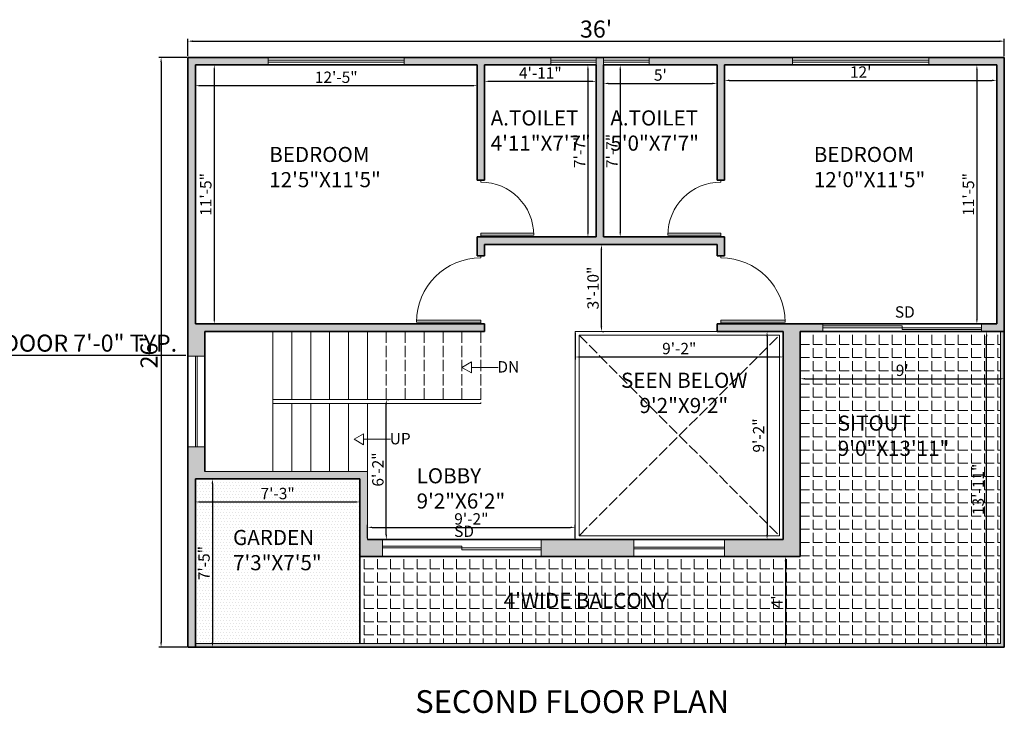
# Model space of a CAD drawing. Units: inches. Extents: x 1947 to 4744, y 610 to 1869.
# Tile 5 of 8: x 4199 to 4720, y 707 to 1074. Entities that reach past the tile are written whole.
import ezdxf

# ---------------------------------------------------------------- set-up
doc = ezdxf.new("R2010")
doc.units = ezdxf.units.IN
doc.linetypes.add('ACAD_ISO02W100', pattern=[15, 12, -3])
for name, color, linetype, lineweight in [('A-ANNO-DIMS', 2, 'Continuous', 18), ('A-ANNO-SYMB', 2, 'Continuous', 18), ('A-ANNO-TEXT', 7, 'Continuous', 18), ('A-ANNO-TITL', 7, 'Continuous', 35), ('A-AREA-IDEN', 7, 'Continuous', 18), ('A-DOOR', 3, 'Continuous', 18), ('A-FLOR-OPEN', 7, 'Continuous', 18), ('A-FLOR-OPEN-PROJ', 8, 'ACAD_ISO02W100', 13), ('A-FLOR-STRS', 7, 'Continuous', 18), ('A-FLOR-STRS-OVHD', 7, 'ACAD_ISO02W100', 13), ('A-GLAZ', 4, 'Continuous', 18), ('A-WALL', 7, 'Continuous', 35), ('A-WALL-PRHT', 7, 'Continuous', 18), ('L-PLNT-PATT', 3, 'Continuous', 13)]:
    doc.layers.add(name, color=color, linetype=linetype, lineweight=lineweight)
doc.layers.add('A-FLOR-PATT', color=251, linetype='Continuous', lineweight=13, true_color=0x636466)
doc.layers.add('A-WALL-PATT', color=18, linetype='Continuous', lineweight=13, true_color=0x000000)
doc.styles.get("Standard").update_dxf_attribs({"font": 'arial.ttf'})
doc.dimstyles.new('ISO-25', dxfattribs={"dimtxt": 9, "dimasz": 2.5, "dimexe": 1.25, "dimexo": 0.625, "dimtad": 1, "dimdec": 1, "dimlunit": 3, "dimtxsty": 'Standard', "dimcen": 2.5, "dimadec": 0, "dimazin": 0, "dimtfac": 1, "dimtdec": 1, "dimtmove": 0, "dimatfit": 3, "dimfxl": 1, "dimarcsym": 0})

# ---------------------------------------------------------------- blocks, each defined once
blk = doc.blocks.new('2')
for p, q in [((4319.45, 1679.18), (4319.45, 1713.18)), ((4320.45, 1679.18), (4320.45, 1713.18)), ((4318.45, 1679.18), (4320.45, 1679.18)), ((4353.45, 1679.18), (4354.45, 1679.18))]:
    blk.add_line(p, q)
at = {"ltscale": 0.5}
blk.add_arc((4319.45, 1679.18), 34, 0, 90, dxfattribs=at)
blk = doc.blocks.new('4')
for p, q in [((3808.6, 1693.11), (3808.6, 1721.11)), ((3809.6, 1693.11), (3809.6, 1721.11)), ((3807.6, 1693.11), (3809.6, 1693.11)), ((3836.6, 1693.11), (3837.6, 1693.11))]:
    blk.add_line(p, q)
at = {"ltscale": 0.5}
blk.add_arc((3808.6, 1693.11), 28, 0, 90, dxfattribs=at)
blk = doc.blocks.new('*D15')
at = {"layer": 'A-ANNO-DIMS', "color": 0, "lineweight": -2, "transparency": 16777216}
for p, q in [((4288.19, 1054.49), (4288.19, 1063.69)), ((4720.19, 1054.49), (4720.19, 1063.69)), ((4290.69, 1062.44), (4717.69, 1062.44))]:
    blk.add_line(p, q, dxfattribs=at)
at = {"layer": 'A-ANNO-DIMS', "color": 0, "transparency": 16777216}
for points in [[(4290.69, 1062.86), (4290.69, 1062.02), (4288.19, 1062.44)], [(4717.69, 1062.86), (4717.69, 1062.02), (4720.19, 1062.44)]]:
    blk.add_solid(points, dxfattribs=at)
at = {"layer": 'Defpoints', "color": 0, "transparency": 16777216}
for p in [(4720.19, 1062.44), (4288.19, 1053.87), (4720.19, 1053.87)]:
    blk.add_point(p, dxfattribs=at)
at = {"layer": 'A-ANNO-DIMS', "color": 0, "transparency": 16777216, "insert": (4504.19, 1067.66), "char_height": 9, "attachment_point": 5}
blk.add_mtext("36'", dxfattribs=at)
blk = doc.blocks.new('*D16')
at = {"layer": 'A-ANNO-DIMS', "color": 0, "lineweight": -2, "transparency": 16777216}
for p, q in [((4287.57, 1053.87), (4272.77, 1053.87)), ((4274.02, 1051.37), (4274.02, 744.37)), ((4287.57, 741.87), (4272.77, 741.87))]:
    blk.add_line(p, q, dxfattribs=at)
at = {"layer": 'A-ANNO-DIMS', "color": 0, "transparency": 16777216}
for points in [[(4273.6, 1051.37), (4274.44, 1051.37), (4274.02, 1053.87)], [(4273.6, 744.37), (4274.44, 744.37), (4274.02, 741.87)]]:
    blk.add_solid(points, dxfattribs=at)
at = {"layer": 'Defpoints', "color": 0, "transparency": 16777216}
for p in [(4288.19, 1053.87), (4274.02, 741.87), (4288.19, 741.87)]:
    blk.add_point(p, dxfattribs=at)
at = {"layer": 'A-ANNO-DIMS', "color": 0, "transparency": 16777216, "insert": (4268.8, 897.87), "char_height": 9, "attachment_point": 5, "rotation": 90}
blk.add_mtext("26'", dxfattribs=at)
blk = doc.blocks.new('*D46')
at = {"layer": 'A-ANNO-DIMS', "color": 0, "lineweight": -2, "transparency": 16777216}
for p, q in [((4292.19, 1049.24), (4292.19, 1037.64)), ((4441.19, 1049.24), (4441.19, 1037.64)), ((4438.69, 1038.89), (4294.69, 1038.89))]:
    blk.add_line(p, q, dxfattribs=at)
at = {"layer": 'A-ANNO-DIMS', "color": 0, "transparency": 16777216}
for points in [[(4294.69, 1039.31), (4294.69, 1038.48), (4292.19, 1038.89)], [(4438.69, 1039.31), (4438.69, 1038.48), (4441.19, 1038.89)]]:
    blk.add_solid(points, dxfattribs=at)
at = {"layer": 'Defpoints', "color": 0, "transparency": 16777216}
for p in [(4292.19, 1049.87), (4441.19, 1049.87), (4292.19, 1038.89)]:
    blk.add_point(p, dxfattribs=at)
at = {"layer": 'A-ANNO-DIMS', "color": 0, "transparency": 16777216, "insert": (4366.69, 1042.58), "char_height": 6, "attachment_point": 5}
blk.add_mtext('12\'-5"', dxfattribs=at)
blk = doc.blocks.new('*D47')
at = {"layer": 'A-ANNO-DIMS', "color": 0, "lineweight": -2, "transparency": 16777216}
for p, q in [((4292.82, 1049.87), (4303.4, 1049.87)), ((4302.15, 1047.37), (4302.15, 915.37)), ((4292.82, 912.87), (4303.4, 912.87))]:
    blk.add_line(p, q, dxfattribs=at)
at = {"layer": 'A-ANNO-DIMS', "color": 0, "transparency": 16777216}
for points in [[(4301.74, 1047.37), (4302.57, 1047.37), (4302.15, 1049.87)], [(4301.74, 915.37), (4302.57, 915.37), (4302.15, 912.87)]]:
    blk.add_solid(points, dxfattribs=at)
at = {"layer": 'Defpoints', "color": 0, "transparency": 16777216}
for p in [(4292.19, 1049.87), (4292.19, 912.87), (4302.15, 912.87)]:
    blk.add_point(p, dxfattribs=at)
at = {"layer": 'A-ANNO-DIMS', "color": 0, "transparency": 16777216, "insert": (4298.46, 981.37), "char_height": 6, "attachment_point": 5, "rotation": 90}
blk.add_mtext('11\'-5"', dxfattribs=at)
blk = doc.blocks.new('*D48')
at = {"layer": 'A-ANNO-DIMS', "color": 0, "lineweight": -2, "transparency": 16777216}
for p, q in [((4445.19, 1049.24), (4445.19, 1039.95)), ((4504.19, 1049.24), (4504.19, 1039.95)), ((4447.69, 1041.2), (4501.69, 1041.2))]:
    blk.add_line(p, q, dxfattribs=at)
at = {"layer": 'A-ANNO-DIMS', "color": 0, "transparency": 16777216}
for points in [[(4447.69, 1041.61), (4447.69, 1040.78), (4445.19, 1041.2)], [(4501.69, 1041.61), (4501.69, 1040.78), (4504.19, 1041.2)]]:
    blk.add_solid(points, dxfattribs=at)
at = {"layer": 'Defpoints', "color": 0, "transparency": 16777216}
for p in [(4445.19, 1049.87), (4504.19, 1049.87), (4504.19, 1041.2)]:
    blk.add_point(p, dxfattribs=at)
at = {"layer": 'A-ANNO-DIMS', "color": 0, "transparency": 16777216, "insert": (4474.69, 1044.83), "char_height": 6, "attachment_point": 5}
blk.add_mtext('4\'-11"', dxfattribs=at)
blk = doc.blocks.new('*D49')
at = {"layer": 'A-ANNO-DIMS', "color": 0, "lineweight": -2, "transparency": 16777216}
for p, q in [((4503.57, 1049.87), (4498.62, 1049.87)), ((4499.87, 1047.37), (4499.87, 961.37)), ((4503.57, 958.87), (4498.62, 958.87))]:
    blk.add_line(p, q, dxfattribs=at)
at = {"layer": 'A-ANNO-DIMS', "color": 0, "transparency": 16777216}
for points in [[(4499.45, 1047.37), (4500.29, 1047.37), (4499.87, 1049.87)], [(4499.45, 961.37), (4500.29, 961.37), (4499.87, 958.87)]]:
    blk.add_solid(points, dxfattribs=at)
at = {"layer": 'Defpoints', "color": 0, "transparency": 16777216}
for p in [(4504.19, 1049.87), (4499.87, 958.87), (4504.19, 958.87)]:
    blk.add_point(p, dxfattribs=at)
at = {"layer": 'A-ANNO-DIMS', "color": 0, "transparency": 16777216, "insert": (4496.25, 1004.37), "char_height": 6, "attachment_point": 5, "rotation": 90}
blk.add_mtext('7\'-7"', dxfattribs=at)
blk = doc.blocks.new('*D50')
at = {"layer": 'A-ANNO-DIMS', "color": 0, "lineweight": -2, "transparency": 16777216}
for p, q in [((4508.19, 1049.24), (4508.19, 1038.83)), ((4568.19, 1049.24), (4568.19, 1038.83)), ((4510.69, 1040.08), (4565.69, 1040.08))]:
    blk.add_line(p, q, dxfattribs=at)
at = {"layer": 'A-ANNO-DIMS', "color": 0, "transparency": 16777216}
for points in [[(4510.69, 1040.49), (4510.69, 1039.66), (4508.19, 1040.08)], [(4565.69, 1040.49), (4565.69, 1039.66), (4568.19, 1040.08)]]:
    blk.add_solid(points, dxfattribs=at)
at = {"layer": 'Defpoints', "color": 0, "transparency": 16777216}
for p in [(4508.19, 1049.87), (4568.19, 1049.87), (4568.19, 1040.08)]:
    blk.add_point(p, dxfattribs=at)
at = {"layer": 'A-ANNO-DIMS', "color": 0, "transparency": 16777216, "insert": (4538.19, 1043.75), "char_height": 6, "attachment_point": 5}
blk.add_mtext("5'", dxfattribs=at)
blk = doc.blocks.new('*D51')
at = {"layer": 'A-ANNO-DIMS', "color": 0, "lineweight": -2, "transparency": 16777216}
for p, q in [((4508.82, 1049.87), (4518.2, 1049.87)), ((4516.95, 1047.37), (4516.95, 961.37)), ((4508.82, 958.87), (4518.2, 958.87))]:
    blk.add_line(p, q, dxfattribs=at)
at = {"layer": 'A-ANNO-DIMS', "color": 0, "transparency": 16777216}
for points in [[(4516.54, 1047.37), (4517.37, 1047.37), (4516.95, 1049.87)], [(4516.54, 961.37), (4517.37, 961.37), (4516.95, 958.87)]]:
    blk.add_solid(points, dxfattribs=at)
at = {"layer": 'Defpoints', "color": 0, "transparency": 16777216}
for p in [(4508.19, 1049.87), (4508.19, 958.87), (4516.95, 958.87)]:
    blk.add_point(p, dxfattribs=at)
at = {"layer": 'A-ANNO-DIMS', "color": 0, "transparency": 16777216, "insert": (4513.33, 1004.37), "char_height": 6, "attachment_point": 5, "rotation": 90}
blk.add_mtext('7\'-7"', dxfattribs=at)
blk = doc.blocks.new('*D52')
at = {"layer": 'A-ANNO-DIMS', "color": 0, "lineweight": -2, "transparency": 16777216}
for p, q in [((4572.19, 1049.24), (4572.19, 1040.44)), ((4716.19, 1049.24), (4716.19, 1040.44)), ((4574.69, 1041.69), (4713.69, 1041.69))]:
    blk.add_line(p, q, dxfattribs=at)
at = {"layer": 'A-ANNO-DIMS', "color": 0, "transparency": 16777216}
for points in [[(4574.69, 1042.11), (4574.69, 1041.27), (4572.19, 1041.69)], [(4713.69, 1042.11), (4713.69, 1041.27), (4716.19, 1041.69)]]:
    blk.add_solid(points, dxfattribs=at)
at = {"layer": 'Defpoints', "color": 0, "transparency": 16777216}
for p in [(4572.19, 1049.87), (4716.19, 1049.87), (4716.19, 1041.69)]:
    blk.add_point(p, dxfattribs=at)
at = {"layer": 'A-ANNO-DIMS', "color": 0, "transparency": 16777216, "insert": (4644.19, 1045.33), "char_height": 6, "attachment_point": 5}
blk.add_mtext("12'", dxfattribs=at)
blk = doc.blocks.new('*D53')
at = {"layer": 'A-ANNO-DIMS', "color": 0, "lineweight": -2, "transparency": 16777216}
for p, q in [((4715.57, 1049.87), (4704.43, 1049.87)), ((4705.68, 1047.37), (4705.68, 915.37)), ((4715.57, 912.87), (4704.43, 912.87))]:
    blk.add_line(p, q, dxfattribs=at)
at = {"layer": 'A-ANNO-DIMS', "color": 0, "transparency": 16777216}
for points in [[(4705.26, 1047.37), (4706.1, 1047.37), (4705.68, 1049.87)], [(4705.26, 915.37), (4706.1, 915.37), (4705.68, 912.87)]]:
    blk.add_solid(points, dxfattribs=at)
at = {"layer": 'Defpoints', "color": 0, "transparency": 16777216}
for p in [(4716.19, 1049.87), (4705.68, 912.87), (4716.19, 912.87)]:
    blk.add_point(p, dxfattribs=at)
at = {"layer": 'A-ANNO-DIMS', "color": 0, "transparency": 16777216, "insert": (4701.99, 981.37), "char_height": 6, "attachment_point": 5, "rotation": 90}
blk.add_mtext('11\'-5"', dxfattribs=at)
blk = doc.blocks.new('*D54')
at = {"layer": 'A-ANNO-DIMS', "color": 0, "lineweight": -2, "transparency": 16777216}
for p, q in [((4292.19, 823.5), (4292.19, 817.44)), ((4379.19, 823.5), (4379.19, 817.44)), ((4294.69, 818.69), (4376.69, 818.69))]:
    blk.add_line(p, q, dxfattribs=at)
at = {"layer": 'A-ANNO-DIMS', "color": 0, "transparency": 16777216}
for points in [[(4294.69, 819.11), (4294.69, 818.28), (4292.19, 818.69)], [(4376.69, 819.11), (4376.69, 818.28), (4379.19, 818.69)]]:
    blk.add_solid(points, dxfattribs=at)
at = {"layer": 'Defpoints', "color": 0, "transparency": 16777216}
for p in [(4292.19, 824.13), (4379.19, 824.13), (4379.19, 818.69)]:
    blk.add_point(p, dxfattribs=at)
at = {"layer": 'A-ANNO-DIMS', "color": 0, "transparency": 16777216, "insert": (4335.69, 822.38), "char_height": 6, "attachment_point": 5}
blk.add_mtext('7\'-3"', dxfattribs=at)
blk = doc.blocks.new('*D55')
at = {"layer": 'A-ANNO-DIMS', "color": 0, "lineweight": -2, "transparency": 16777216}
for p, q in [((4301.81, 830.87), (4302.44, 830.87)), ((4301.19, 828.37), (4301.19, 744.37)), ((4301.81, 741.87), (4302.44, 741.87))]:
    blk.add_line(p, q, dxfattribs=at)
at = {"layer": 'A-ANNO-DIMS', "color": 0, "transparency": 16777216}
for points in [[(4300.77, 828.37), (4301.6, 828.37), (4301.19, 830.87)], [(4300.77, 744.37), (4301.6, 744.37), (4301.19, 741.87)]]:
    blk.add_solid(points, dxfattribs=at)
at = {"layer": 'Defpoints', "color": 0, "transparency": 16777216}
for p in [(4301.19, 830.87), (4301.19, 741.87), (4301.19, 741.87)]:
    blk.add_point(p, dxfattribs=at)
at = {"layer": 'A-ANNO-DIMS', "color": 0, "transparency": 16777216, "insert": (4297.51, 786.37), "char_height": 6, "attachment_point": 5, "rotation": 90}
blk.add_mtext('7\'-5"', dxfattribs=at)
blk = doc.blocks.new('*D56')
at = {"layer": 'A-ANNO-DIMS', "color": 0, "lineweight": -2, "transparency": 16777216}
for p, q in [((4383.19, 799.49), (4383.19, 806.52)), ((4385.69, 805.27), (4490.69, 805.27)), ((4493.19, 799.49), (4493.19, 806.52))]:
    blk.add_line(p, q, dxfattribs=at)
at = {"layer": 'A-ANNO-DIMS', "color": 0, "transparency": 16777216}
for points in [[(4385.69, 805.69), (4385.69, 804.85), (4383.19, 805.27)], [(4490.69, 805.69), (4490.69, 804.85), (4493.19, 805.27)]]:
    blk.add_solid(points, dxfattribs=at)
at = {"layer": 'Defpoints', "color": 0, "transparency": 16777216}
for p in [(4493.19, 805.27), (4383.19, 798.87), (4493.19, 798.87)]:
    blk.add_point(p, dxfattribs=at)
at = {"layer": 'A-ANNO-DIMS', "color": 0, "transparency": 16777216, "insert": (4438.19, 808.96), "char_height": 6, "attachment_point": 5}
blk.add_mtext('9\'-2"', dxfattribs=at)
blk = doc.blocks.new('*D57')
at = {"layer": 'A-ANNO-DIMS', "color": 0, "lineweight": -2, "transparency": 16777216}
for p, q in [((4393.19, 801.37), (4393.19, 870.37)), ((4393.82, 872.87), (4394.44, 872.87)), ((4391.82, 798.87), (4394.44, 798.87))]:
    blk.add_line(p, q, dxfattribs=at)
at = {"layer": 'A-ANNO-DIMS', "color": 0, "transparency": 16777216}
for points in [[(4392.78, 870.37), (4393.61, 870.37), (4393.19, 872.87)], [(4392.78, 801.37), (4393.61, 801.37), (4393.19, 798.87)]]:
    blk.add_solid(points, dxfattribs=at)
at = {"layer": 'Defpoints', "color": 0, "transparency": 16777216}
for p in [(4393.19, 872.87), (4393.19, 872.87), (4391.19, 798.87)]:
    blk.add_point(p, dxfattribs=at)
at = {"layer": 'A-ANNO-DIMS', "color": 0, "transparency": 16777216, "insert": (4389.5, 835.87), "char_height": 6, "attachment_point": 5, "rotation": 90}
blk.add_mtext('6\'-2"', dxfattribs=at)
blk = doc.blocks.new('*D58')
at = {"layer": 'A-ANNO-DIMS', "color": 0, "lineweight": -2, "transparency": 16777216}
for p, q in [((4507.65, 954.87), (4508.28, 954.87)), ((4507.03, 911.37), (4507.03, 952.37)), ((4507.65, 908.87), (4508.28, 908.87))]:
    blk.add_line(p, q, dxfattribs=at)
at = {"layer": 'A-ANNO-DIMS', "color": 0, "transparency": 16777216}
for points in [[(4506.61, 952.37), (4507.44, 952.37), (4507.03, 954.87)], [(4506.61, 911.37), (4507.44, 911.37), (4507.03, 908.87)]]:
    blk.add_solid(points, dxfattribs=at)
at = {"layer": 'Defpoints', "color": 0, "transparency": 16777216}
for p in [(4507.03, 954.87), (4507.03, 954.87), (4507.03, 908.87)]:
    blk.add_point(p, dxfattribs=at)
at = {"layer": 'A-ANNO-DIMS', "color": 0, "transparency": 16777216, "insert": (4503.34, 931.87), "char_height": 6, "attachment_point": 5, "rotation": 90}
blk.add_mtext('3\'-10"', dxfattribs=at)
blk = doc.blocks.new('*D59')
at = {"layer": 'A-ANNO-DIMS', "color": 0, "lineweight": -2, "transparency": 16777216}
for p, q in [((4493.19, 908.24), (4493.19, 894.14)), ((4603.19, 908.24), (4603.19, 894.14)), ((4495.69, 895.39), (4600.69, 895.39))]:
    blk.add_line(p, q, dxfattribs=at)
at = {"layer": 'A-ANNO-DIMS', "color": 0, "transparency": 16777216}
for points in [[(4495.69, 895.8), (4495.69, 894.97), (4493.19, 895.39)], [(4600.69, 895.8), (4600.69, 894.97), (4603.19, 895.39)]]:
    blk.add_solid(points, dxfattribs=at)
at = {"layer": 'Defpoints', "color": 0, "transparency": 16777216}
for p in [(4493.19, 908.87), (4603.19, 908.87), (4603.19, 895.39)]:
    blk.add_point(p, dxfattribs=at)
at = {"layer": 'A-ANNO-DIMS', "color": 0, "transparency": 16777216, "insert": (4548.19, 899.08), "char_height": 6, "attachment_point": 5}
blk.add_mtext('9\'-2"', dxfattribs=at)
blk = doc.blocks.new('*D60')
at = {"layer": 'A-ANNO-DIMS', "color": 0, "lineweight": -2, "transparency": 16777216}
for p, q in [((4602.57, 908.87), (4593.42, 908.87)), ((4594.67, 906.37), (4594.67, 801.37)), ((4602.57, 798.87), (4593.42, 798.87))]:
    blk.add_line(p, q, dxfattribs=at)
at = {"layer": 'A-ANNO-DIMS', "color": 0, "transparency": 16777216}
for points in [[(4594.25, 906.37), (4595.08, 906.37), (4594.67, 908.87)], [(4594.25, 801.37), (4595.08, 801.37), (4594.67, 798.87)]]:
    blk.add_solid(points, dxfattribs=at)
at = {"layer": 'Defpoints', "color": 0, "transparency": 16777216}
for p in [(4603.19, 908.87), (4594.67, 798.87), (4603.19, 798.87)]:
    blk.add_point(p, dxfattribs=at)
at = {"layer": 'A-ANNO-DIMS', "color": 0, "transparency": 16777216, "insert": (4590.98, 853.87), "char_height": 6, "attachment_point": 5, "rotation": 90}
blk.add_mtext('9\'-2"', dxfattribs=at)
blk = doc.blocks.new('*D61')
at = {"layer": 'A-ANNO-DIMS', "color": 0, "lineweight": -2, "transparency": 16777216}
for p, q in [((4612.19, 884.49), (4612.19, 885.12)), ((4614.69, 883.87), (4717.69, 883.87)), ((4720.19, 884.49), (4720.19, 885.12))]:
    blk.add_line(p, q, dxfattribs=at)
at = {"layer": 'A-ANNO-DIMS', "color": 0, "transparency": 16777216}
for points in [[(4614.69, 884.28), (4614.69, 883.45), (4612.19, 883.87)], [(4717.69, 884.28), (4717.69, 883.45), (4720.19, 883.87)]]:
    blk.add_solid(points, dxfattribs=at)
at = {"layer": 'Defpoints', "color": 0, "transparency": 16777216}
for p in [(4612.19, 883.87), (4720.19, 883.87), (4720.19, 883.87)]:
    blk.add_point(p, dxfattribs=at)
at = {"layer": 'A-ANNO-DIMS', "color": 0, "transparency": 16777216, "insert": (4666.19, 887.56), "char_height": 6, "attachment_point": 5}
blk.add_mtext("9'", dxfattribs=at)
blk = doc.blocks.new('*D62')
at = {"layer": 'A-ANNO-DIMS', "color": 0, "lineweight": -2, "transparency": 16777216}
for p, q in [((4611.57, 789.87), (4603.14, 789.87)), ((4604.39, 787.37), (4604.39, 744.37)), ((4611.57, 741.87), (4603.14, 741.87))]:
    blk.add_line(p, q, dxfattribs=at)
at = {"layer": 'A-ANNO-DIMS', "color": 0, "transparency": 16777216}
for points in [[(4603.97, 787.37), (4604.8, 787.37), (4604.39, 789.87)], [(4603.97, 744.37), (4604.8, 744.37), (4604.39, 741.87)]]:
    blk.add_solid(points, dxfattribs=at)
at = {"layer": 'Defpoints', "color": 0, "transparency": 16777216}
for p in [(4612.19, 789.87), (4604.39, 741.87), (4612.19, 741.87)]:
    blk.add_point(p, dxfattribs=at)
at = {"layer": 'A-ANNO-DIMS', "color": 0, "transparency": 16777216, "insert": (4600.76, 765.87), "char_height": 6, "attachment_point": 5, "rotation": 90}
blk.add_mtext("4'", dxfattribs=at)
blk = doc.blocks.new('*D63')
at = {"layer": 'A-ANNO-DIMS', "color": 0, "lineweight": -2, "transparency": 16777216}
for p, q in [((4719.57, 908.87), (4709.58, 908.87)), ((4710.83, 744.37), (4710.83, 906.37)), ((4719.57, 741.87), (4709.58, 741.87))]:
    blk.add_line(p, q, dxfattribs=at)
at = {"layer": 'A-ANNO-DIMS', "color": 0, "transparency": 16777216}
for points in [[(4710.42, 906.37), (4711.25, 906.37), (4710.83, 908.87)], [(4710.42, 744.37), (4711.25, 744.37), (4710.83, 741.87)]]:
    blk.add_solid(points, dxfattribs=at)
at = {"layer": 'Defpoints', "color": 0, "transparency": 16777216}
for p in [(4710.83, 908.87), (4720.19, 908.87), (4720.19, 741.87)]:
    blk.add_point(p, dxfattribs=at)
at = {"layer": 'A-ANNO-DIMS', "color": 0, "transparency": 16777216, "insert": (4707.14, 825.37), "char_height": 6, "attachment_point": 5, "rotation": 90}
blk.add_mtext('13\'-11"', dxfattribs=at)
blk = doc.blocks.new('WIN-72-4')
for p, q in [((0, 0), (0, 4)), ((72, 2.5), (0, 2.5)), ((72, 1.5), (0, 1.5)), ((72, 0), (72, 4))]:
    blk.add_line(p, q)
blk = doc.blocks.new('WIN-48-9')
for p, q in [((0, 0), (0, 9)), ((48, 0), (48, 9)), ((48, 5), (0, 5)), ((48, 4), (0, 4))]:
    blk.add_line(p, q)
blk = doc.blocks.new('WIN-24-4')
for p, q in [((0, 0), (0, 4)), ((24, 2.5), (0, 2.5)), ((24, 1.5), (0, 1.5)), ((24, 0), (24, 4))]:
    blk.add_line(p, q)
blk = doc.blocks.new('DOOR-SLIDE-84-4')
for p, q in [((0, 0), (0, 4)), ((42, 3), (0, 3)), ((0, 2), (84, 2)), ((42, 2), (42, 3)), ((42, 2), (42, 1)), ((42, 1), (84, 1)), ((84, 0), (84, 4))]:
    blk.add_line(p, q)
blk = doc.blocks.new('STAIR-DIRECTION')
blk.add_line((2.91, 14.18), (2.91, 0))
blk.add_lwpolyline([(2.91, 19.23), (0, 14.18), (5.83, 14.18)], close=True)
blk = doc.blocks.new('*D92')
at = {"layer": 'A-ANNO-DIMS', "color": 0, "lineweight": -2, "transparency": 16777216}
for p, q in [((4049.53, 908.24), (4049.53, 895.02)), ((4133.53, 908.24), (4133.53, 895.02)), ((4052.03, 896.27), (4131.03, 896.27)), ((4133.53, 896.27), (4287.11, 896.27))]:
    blk.add_line(p, q, dxfattribs=at)
at = {"layer": 'A-ANNO-DIMS', "color": 0, "transparency": 16777216}
for points in [[(4052.03, 896.68), (4052.03, 895.85), (4049.53, 896.27)], [(4131.03, 896.68), (4131.03, 895.85), (4133.53, 896.27)]]:
    blk.add_solid(points, dxfattribs=at)
at = {"layer": 'Defpoints', "color": 0, "transparency": 16777216}
for p in [(4049.53, 908.87), (4133.53, 908.87), (4133.53, 896.27)]:
    blk.add_point(p, dxfattribs=at)
at = {"layer": 'A-ANNO-DIMS', "color": 0, "transparency": 16777216, "insert": (4211.57, 901.55), "char_height": 9, "attachment_point": 5}
blk.add_mtext('SLIDING DOOR 7\'-0" TYP.', dxfattribs=at)

msp = doc.modelspace()

# ---------------------------------------------------------------- hatches: boundary and pattern name
at = {"layer": 'A-FLOR-PATT'}
h = msp.add_hatch(dxfattribs=at)
h.set_pattern_fill('ANGLE', color=256)
h.set_pattern_definition([(0, (574.662, -6.012), (0, 6.985), [5.08, -1.905]), (90, (574.662, -6.012), (-6.985, 4e-16), [5.08, -1.905])])
h.paths.add_polyline_path([(4718.19, 743.87), (4718.19, 908.87), (4612.19, 908.87), (4612.19, 789.87), (4379.19, 789.87), (4379.19, 743.87)])
h.paths.add_polyline_path([(4453.14, 758.1), (4556.05, 758.1), (4556.05, 775.18), (4453.14, 775.18)], flags=24)
h.paths.add_polyline_path([(4629.35, 838.52), (4691.49, 838.52), (4691.49, 868.94), (4629.35, 868.94)], flags=24)
at = {"layer": 'A-WALL-PATT'}
h = msp.add_hatch(color=256, dxfattribs=at)
h.dxf.hatch_style = 1
h.paths.add_polyline_path([(4508.19, 1049.87), (4508.19, 1053.87), (4504.19, 1053.87), (4504.19, 1049.87), (4504.19, 958.87), (4441.19, 958.87), (4441.19, 948.87), (4445.19, 948.87), (4445.19, 954.87), (4568.19, 954.87), (4568.19, 948.87), (4572.19, 948.87), (4572.19, 958.87), (4508.19, 958.87)])
h.paths.add_polyline_path([(4608.19, 1053.87), (4532.19, 1053.87), (4532.19, 1049.87), (4568.19, 1049.87), (4568.19, 988.87), (4572.19, 988.87), (4572.19, 1049.87), (4608.19, 1049.87)])
h.paths.add_polyline_path([(4480.19, 1053.87), (4402.69, 1053.87), (4402.69, 1049.87), (4441.19, 1049.87), (4441.19, 988.87), (4445.19, 988.87), (4445.19, 1049.87), (4480.19, 1049.87)])
h.paths.add_polyline_path([(4720.19, 1053.87), (4680.19, 1053.87), (4680.19, 1049.87), (4716.19, 1049.87), (4716.19, 912.87), (4708.19, 912.87), (4708.19, 908.87), (4720.19, 908.87)])
h.paths.add_polyline_path([(4612.19, 908.87), (4624.19, 908.87), (4624.19, 912.87), (4568.19, 912.87), (4568.19, 908.87), (4603.19, 908.87), (4603.19, 798.87), (4572.19, 798.87), (4572.19, 789.87), (4612.19, 789.87)])
h.paths.add_polyline_path([(4524.19, 798.87), (4475.19, 798.87), (4475.19, 789.87), (4524.19, 789.87)], flags=17)
h.paths.add_polyline_path([(4391.19, 798.87), (4383.19, 798.87), (4383.19, 834.87), (4297.19, 834.87), (4297.19, 847.87), (4288.19, 847.87), (4288.19, 741.87), (4292.19, 741.87), (4292.19, 830.87), (4379.19, 830.87), (4379.19, 789.87), (4391.19, 789.87)])
h.paths.add_polyline_path([(4297.19, 908.87), (4445.19, 908.87), (4445.19, 912.87), (4292.19, 912.87), (4292.19, 1049.87), (4330.69, 1049.87), (4330.69, 1053.87), (4288.19, 1053.87), (4288.19, 895.87), (4297.19, 895.87)])
h.paths.add_polyline_path([(4720.19, 908.87), (4718.19, 908.87), (4718.19, 743.87), (4292.19, 743.87), (4292.19, 741.87), (4720.19, 741.87)])
at = {"layer": 'L-PLNT-PATT'}
h = msp.add_hatch(dxfattribs=at)
h.set_pattern_fill('DOTS', color=256)
h.set_pattern_definition([(0, (574.6621, -6.0122), (0.79375, 1.5875), [0, -1.5875])])
h.paths.add_polyline_path([(4379.19, 743.87), (4379.19, 830.87), (4292.19, 830.87), (4292.19, 743.87)])
h.paths.add_polyline_path([(4309.64, 778.03), (4362.88, 778.03), (4362.88, 808.45), (4309.64, 808.45)], flags=24)

# ---------------------------------------------------------------- linework, layer by layer
at = {"layer": 'A-DOOR'}
for p, q in [((4391.19, 798.87), (4391.19, 789.87)), ((4475.19, 798.87), (4475.19, 789.87)), ((4433.19, 795.37), (4391.19, 795.37)), ((4391.19, 794.37), (4475.19, 794.37)), ((4433.19, 794.37), (4433.19, 795.37)), ((4433.19, 794.37), (4433.19, 793.37)), ((4433.19, 793.37), (4475.19, 793.37))]:
    msp.add_line(p, q, dxfattribs=at)
at = {"layer": 'A-FLOR-OPEN'}
for points in [[(4603.19, 798.87), (4493.19, 798.87), (4493.19, 908.87), (4603.19, 908.87)], [(4601.19, 800.87), (4495.19, 800.87), (4495.19, 906.87), (4601.19, 906.87)]]:
    msp.add_lwpolyline(points, close=True, dxfattribs=at)
at = {"layer": 'A-FLOR-OPEN-PROJ', "ltscale": 0.5}
for p, q in [((4495.19, 906.87), (4601.19, 800.87)), ((4495.19, 800.87), (4601.19, 906.87))]:
    msp.add_line(p, q, dxfattribs=at)
at = {"layer": 'A-FLOR-STRS'}
for p, q in [((4333.19, 908.87), (4333.19, 834.87)), ((4343.19, 908.87), (4343.19, 872.87)), ((4353.19, 908.87), (4353.19, 872.87)), ((4363.19, 908.87), (4363.19, 872.87)), ((4373.19, 908.87), (4373.19, 872.87)), ((4383.19, 908.87), (4383.19, 872.87)), ((4443.19, 872.87), (4333.19, 872.87)), ((4333.19, 870.87), (4443.19, 870.87)), ((4343.19, 870.87), (4343.19, 834.87)), ((4353.19, 870.87), (4353.19, 834.87)), ((4363.19, 870.87), (4363.19, 834.87)), ((4373.19, 870.87), (4373.19, 834.87)), ((4383.19, 870.87), (4383.19, 798.87)), ((4297.19, 834.87), (4383.19, 834.87))]:
    msp.add_line(p, q, dxfattribs=at)
at = {"layer": 'A-FLOR-STRS-OVHD', "ltscale": 0.5}
for p, q in [((4393.19, 908.87), (4393.19, 872.87)), ((4403.19, 908.87), (4403.19, 872.87)), ((4413.19, 908.87), (4413.19, 872.87)), ((4423.19, 908.87), (4423.19, 872.87)), ((4433.19, 908.87), (4433.19, 872.87)), ((4443.19, 908.87), (4443.19, 870.87))]:
    msp.add_line(p, q, dxfattribs=at)
at = {"layer": 'A-GLAZ'}
for p, q in [((4508.19, 1049.87), (4508.19, 1053.87)), ((4532.19, 1049.87), (4532.19, 1053.87)), ((4532.19, 1052.37), (4508.19, 1052.37)), ((4532.19, 1051.37), (4508.19, 1051.37))]:
    msp.add_line(p, q, dxfattribs=at)
at = {"layer": 'A-WALL'}
for p, q in [((4720.19, 1053.87), (4288.19, 1053.87)), ((4288.19, 1053.87), (4288.19, 741.87)), ((4720.19, 741.87), (4720.19, 1053.87)), ((4441.19, 1049.87), (4292.19, 1049.87)), ((4292.19, 1049.87), (4292.19, 912.87)), ((4441.19, 1049.87), (4441.19, 988.87)), ((4504.19, 1049.87), (4445.19, 1049.87)), ((4445.19, 1049.87), (4445.19, 988.87)), ((4504.19, 958.87), (4504.19, 1049.87)), ((4568.19, 1049.87), (4508.19, 1049.87)), ((4508.19, 958.87), (4508.19, 1049.87)), ((4568.19, 988.87), (4568.19, 1049.87)), ((4716.19, 1049.87), (4572.19, 1049.87)), ((4572.19, 988.87), (4572.19, 1049.87)), ((4716.19, 912.87), (4716.19, 1049.87)), ((4445.19, 988.87), (4441.19, 988.87)), ((4572.19, 988.87), (4568.19, 988.87)), ((4504.19, 958.87), (4441.19, 958.87)), ((4441.19, 958.87), (4441.19, 948.87)), ((4572.19, 958.87), (4508.19, 958.87)), ((4572.19, 948.87), (4572.19, 958.87)), ((4568.19, 954.87), (4445.19, 954.87)), ((4445.19, 954.87), (4445.19, 948.87)), ((4568.19, 948.87), (4568.19, 954.87)), ((4445.19, 948.87), (4441.19, 948.87)), ((4568.19, 948.87), (4572.19, 948.87)), ((4445.19, 912.87), (4292.19, 912.87)), ((4445.19, 912.87), (4445.19, 908.87)), ((4568.19, 912.87), (4716.19, 912.87)), ((4568.19, 908.87), (4568.19, 912.87)), ((4445.19, 908.87), (4297.19, 908.87)), ((4297.19, 908.87), (4297.19, 834.87)), ((4568.19, 908.87), (4603.19, 908.87)), ((4603.19, 798.87), (4603.19, 908.87)), ((4612.19, 789.87), (4612.19, 908.87)), ((4612.19, 908.87), (4720.19, 908.87)), ((4292.19, 830.87), (4292.19, 741.87)), ((4292.19, 830.87), (4379.19, 830.87)), ((4379.19, 830.87), (4379.19, 743.87)), ((4383.19, 798.87), (4603.19, 798.87)), ((4379.19, 789.87), (4612.19, 789.87)), ((4288.19, 741.87), (4720.19, 741.87))]:
    msp.add_line(p, q, dxfattribs=at)
at = {"layer": 'A-WALL-PRHT'}
for p, q in [((4718.19, 743.87), (4718.19, 908.87)), ((4292.19, 743.87), (4718.19, 743.87))]:
    msp.add_line(p, q, dxfattribs=at)

# ---------------------------------------------------------------- block references
at = {"layer": 'A-ANNO-SYMB'}
for p, rotation in [((4452.39, 886.95), 89.99999999999952), ((4395.36, 848.95), 90.00000000000047)]:
    msp.add_blockref('STAIR-DIRECTION', p, dxfattribs=dict(at, rotation=rotation))
at = {"layer": 'A-DOOR', "xscale": -1, "rotation": 270}
for name, p in [('4', (2750.08, -2848.73)), ('2', (2891.01, -3405.59))]:
    msp.add_blockref(name, p, dxfattribs=at)
at = {"layer": 'A-DOOR'}
for name, p, rotation in [('4', (6263.3, -2848.73), 90.00000000000003), ('2', (6122.38, -3405.59), 90.00000000000003), ('DOOR-SLIDE-84-4', (4708.19, 912.87), 180)]:
    msp.add_blockref(name, p, dxfattribs=dict(at, rotation=rotation))
at = {"layer": 'A-GLAZ'}
for name, p in [('WIN-72-4', (4330.69, 1049.87)), ('WIN-72-4', (4608.19, 1049.87)), ('WIN-48-9', (4524.19, 789.87))]:
    msp.add_blockref(name, p, dxfattribs=at)
for name, p, rotation in [('WIN-24-4', (4504.19, 1053.87), 180), ('WIN-48-9', (4297.19, 847.87), 89.9999999999982)]:
    msp.add_blockref(name, p, dxfattribs=dict(at, rotation=rotation))

# ---------------------------------------------------------------- texts
at = {"layer": 'A-ANNO-TEXT', "char_height": 6, "attachment_point": 1}
for s, insert in [('{\\fTimes New Roman|b0|i0|c0|p18;SD}', (4662.29, 922.19)), ('{\\fTimes New Roman|b0|i0|c0|p18;DN}', (4451.97, 893.18)), ('{\\fTimes New Roman|b0|i0|c0|p18;UP}', (4395, 855.18)), ('{\\fTimes New Roman|b0|i0|c0|p18;SD}', (4429.08, 806.2))]:
    msp.add_mtext_dynamic_manual_height_columns(s, width=158.3328, gutter_width=12.5, heights=[0], dxfattribs=dict(at, insert=insert))
at = {"layer": 'A-ANNO-TITL', "insert": (4408.49, 719.13), "char_height": 12, "attachment_point": 1}
msp.add_mtext_dynamic_manual_height_columns('{\\fTimes New Roman|b0|i0|c0|p18;SECOND FLOOR PLAN}', width=253.4596, gutter_width=12.5, heights=[0], dxfattribs=at)
at = {"layer": 'A-AREA-IDEN', "char_height": 8, "attachment_point": 1}
for s, width, insert in [('{\\fTimes New Roman|b0|i0|c0|p18;A.TOILET\\P4\'11"X7\'7"}', 64.3566, (4448.43, 1025.84)), ('{\\fTimes New Roman|b0|i0|c0|p18;A.TOILET\\P5\'0"X7\'7"}', 64.3566, (4511.73, 1025.84)), ('{\\fTimes New Roman|b0|i0|c0|p18;BEDROOM\\P12\'5"X11\'5"}', 64.3566, (4331.24, 1006.52)), ('{\\fTimes New Roman|b0|i0|c0|p18;BEDROOM\\P12\'0"X11\'5"}', 64.3566, (4619.39, 1006.52)), ('{\\fTimes New Roman|b0|i0|c0|p18;SEEN BELOW\\P    9\'2"X9\'2"}', 135.7043, (4517.38, 887.07)), ('{\\fTimes New Roman|b0|i0|c0|p18;SITOUT\\P9\'0"X13\'11"}', 64.3566, (4632.08, 864.41)), ('{\\fTimes New Roman|b0|i0|c0|p18;LOBBY\\P9\'2"X6\'2"}', 64.3566, (4409.22, 836.55)), ('{\\fTimes New Roman|b0|i0|c0|p18;GARDEN\\P7\'3"X7\'5"}', 64.3566, (4312.08, 803.92)), ("{\\fTimes New Roman|b0|i0|c0|p18;4'WIDE BALCONY}", 158.3328, (4455.32, 770.65))]:
    msp.add_mtext_dynamic_manual_height_columns(s, width=width, gutter_width=12.5, heights=[0], dxfattribs=dict(at, insert=insert))

# ---------------------------------------------------------------- dimensions: what is measured, and where the dimension line sits
at = {"layer": 'A-ANNO-DIMS'}
for base, p1, p2, override, picture, middle in [((4720.19, 1062.44), (4288.19, 1053.87), (4720.19, 1053.87), {"dimclrd": 0, "dimclre": 0, "dimclrt": 0}, '*D15', (4504.19, 1067.66)), ((4292.19, 1038.89), (4441.19, 1049.87), (4292.19, 1049.87), {"dimtxt": 6, "dimclrd": 0, "dimclre": 0, "dimclrt": 0}, '*D46', (4366.69, 1042.58)), ((4504.19, 1041.2), (4445.19, 1049.87), (4504.19, 1049.87), {"dimtxt": 6, "dimclrd": 0, "dimclre": 0, "dimclrt": 0}, '*D48', (4474.69, 1044.83)), ((4568.19, 1040.08), (4508.19, 1049.87), (4568.19, 1049.87), {"dimtxt": 6, "dimclrd": 0, "dimclre": 0, "dimclrt": 0}, '*D50', (4538.19, 1043.75)), ((4716.19, 1041.69), (4572.19, 1049.87), (4716.19, 1049.87), {"dimtxt": 6, "dimclrd": 0, "dimclre": 0, "dimclrt": 0}, '*D52', (4644.19, 1045.33)), ((4603.19, 895.39), (4493.19, 908.87), (4603.19, 908.87), {"dimtxt": 6, "dimclrd": 0, "dimclre": 0, "dimclrt": 0}, '*D59', (4548.19, 899.08)), ((4720.19, 883.87), (4612.19, 883.87), (4720.19, 883.87), {"dimtxt": 6, "dimclrd": 0, "dimclre": 0, "dimclrt": 0}, '*D61', (4666.19, 887.56)), ((4379.19, 818.69), (4292.19, 824.13), (4379.19, 824.13), {"dimtxt": 6, "dimclrd": 0, "dimclre": 0, "dimclrt": 0}, '*D54', (4335.69, 822.38)), ((4493.19, 805.27), (4383.19, 798.87), (4493.19, 798.87), {"dimtxt": 6, "dimclrd": 0, "dimclre": 0, "dimclrt": 0}, '*D56', (4438.19, 808.96))]:
    dim = msp.add_linear_dim(base=base, p1=p1, p2=p2, dimstyle='ISO-25', override=override, dxfattribs=at)
    dim.commit()
    dim.dimension.update_dxf_attribs({"geometry": picture, "text_midpoint": middle})
for base, p1, p2, override, picture, middle in [((4274.02, 741.87), (4288.19, 1053.87), (4288.19, 741.87), {"dimclrd": 0, "dimclre": 0, "dimclrt": 0}, '*D16', (4268.8, 897.87)), ((4302.15, 912.87), (4292.19, 1049.87), (4292.19, 912.87), {"dimtxt": 6, "dimclrd": 0, "dimclre": 0, "dimclrt": 0}, '*D47', (4298.46, 981.37)), ((4499.87, 958.87), (4504.19, 1049.87), (4504.19, 958.87), {"dimtxt": 6, "dimclrd": 0, "dimclre": 0, "dimclrt": 0}, '*D49', (4496.25, 1004.37)), ((4516.95, 958.87), (4508.19, 1049.87), (4508.19, 958.87), {"dimtxt": 6, "dimclrd": 0, "dimclre": 0, "dimclrt": 0}, '*D51', (4513.33, 1004.37)), ((4705.68, 912.87), (4716.19, 1049.87), (4716.19, 912.87), {"dimtxt": 6, "dimclrd": 0, "dimclre": 0, "dimclrt": 0}, '*D53', (4701.99, 981.37)), ((4507.03, 954.87), (4507.03, 908.87), (4507.03, 954.87), {"dimtxt": 6, "dimclrd": 0, "dimclre": 0, "dimclrt": 0}, '*D58', (4503.34, 931.87)), ((4594.67, 798.87), (4603.19, 908.87), (4603.19, 798.87), {"dimtxt": 6, "dimclrd": 0, "dimclre": 0, "dimclrt": 0}, '*D60', (4590.98, 853.87)), ((4710.83, 908.87), (4720.19, 741.87), (4720.19, 908.87), {"dimtxt": 6, "dimclrd": 0, "dimclre": 0, "dimclrt": 0}, '*D63', (4707.14, 825.37)), ((4393.19, 872.87), (4391.19, 798.87), (4393.19, 872.87), {"dimtxt": 6, "dimclrd": 0, "dimclre": 0, "dimclrt": 0}, '*D57', (4389.5, 835.87)), ((4301.19, 741.87), (4301.19, 830.87), (4301.19, 741.87), {"dimtxt": 6, "dimclrd": 0, "dimclre": 0, "dimclrt": 0}, '*D55', (4297.51, 786.37)), ((4604.39, 741.87), (4612.19, 789.87), (4612.19, 741.87), {"dimtxt": 6, "dimclrd": 0, "dimclre": 0, "dimclrt": 0}, '*D62', (4600.76, 765.87))]:
    dim = msp.add_linear_dim(base=base, p1=p1, p2=p2, angle=90, dimstyle='ISO-25', override=override, dxfattribs=at)
    dim.commit()
    dim.dimension.update_dxf_attribs({"geometry": picture, "text_midpoint": middle})
dim = msp.add_linear_dim(base=(4133.53, 896.27), p1=(4049.53, 908.87), p2=(4133.53, 908.87), text='SLIDING DOOR <> TYP.', dimstyle='ISO-25', override={"dimdec": 1, "dimlfac": 1, "dimrnd": 0, "dimzin": 1, "dimdsep": 46, "dimlunit": 4, "dimfrac": 2}, dxfattribs=at)
dim.commit()
dim.dimension.update_dxf_attribs({"geometry": '*D92', "text_midpoint": (4211.57, 901.55)})

doc.saveas('drawing.dxf')
